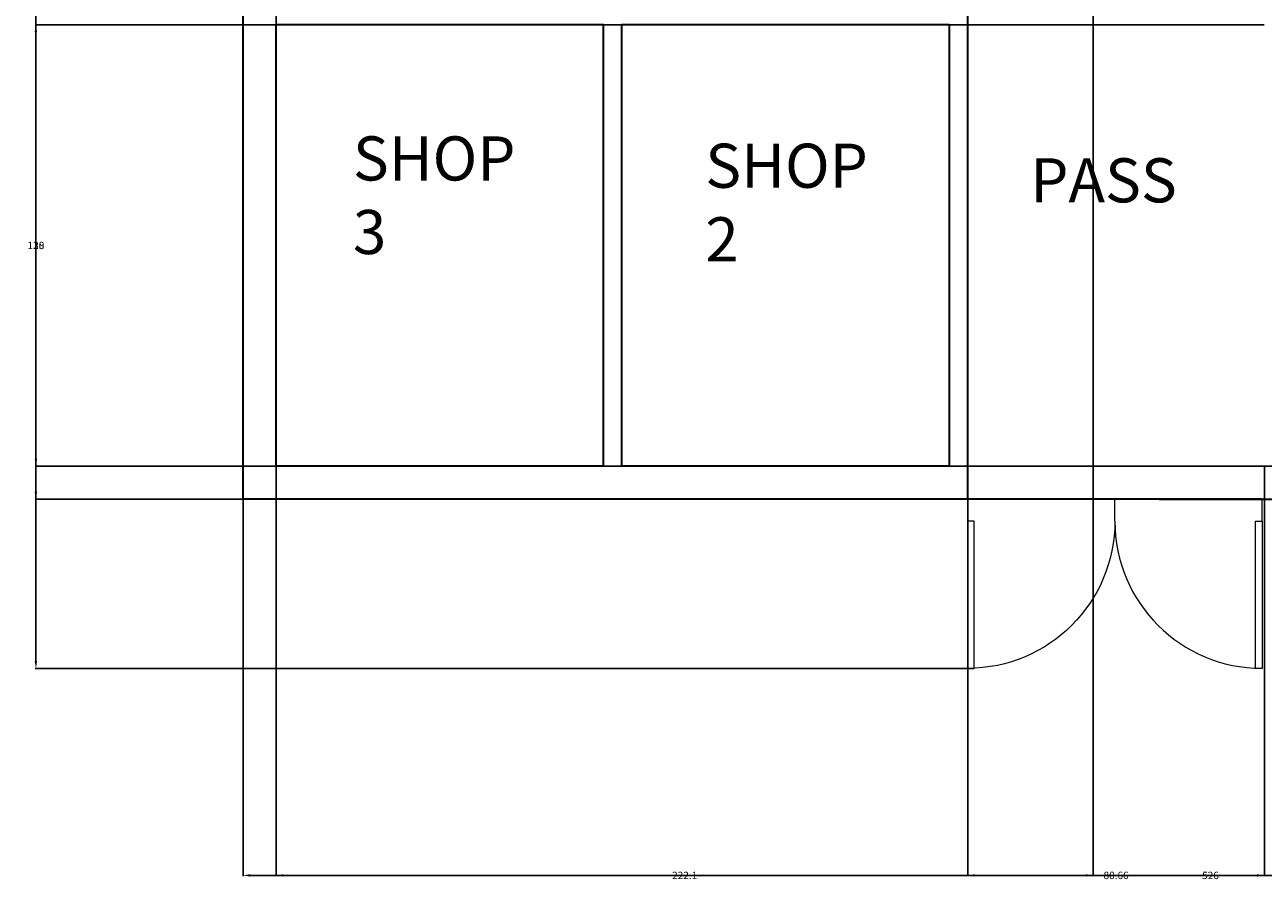
# Model space of a CAD drawing. Units: inches. Extents: x 190 to 836, y -241 to 999.
# Tile 1 of 9: x 191 to 528, y -241 to -8. Entities that reach past the tile are written whole.
import ezdxf

# ---------------------------------------------------------------- set-up
doc = ezdxf.new("R2010")
doc.units = ezdxf.units.IN
doc.header["$MEASUREMENT"] = 0
for name, color, linetype, lineweight in [('A-ANNO-DIMS', 2, 'Continuous', 18), ('A-AREA-IDEN', 7, 'Continuous', 18), ('A-DOOR', 3, 'Continuous', 18), ('A-WALL', 7, 'Continuous', 35)]:
    doc.layers.add(name, color=color, linetype=linetype, lineweight=lineweight)
doc.styles.get("Standard").update_dxf_attribs({"font": 'arial.ttf'})
doc.dimstyles.get("Standard").update_dxf_attribs({"dimtxt": 2, "dimasz": 2, "dimexe": 0.18, "dimexo": 0.0625, "dimgap": 0.09, "dimtad": 0, "dimtih": 1, "dimtoh": 1, "dimdec": 0, "dimzin": 0, "dimdsep": 46, "dimlunit": 3, "dimtxsty": 'Standard', "dimcen": 0.09, "dimadec": 0, "dimazin": 0, "dimtfac": 1, "dimtdec": 0, "dimtofl": 0, "dimtmove": 0, "dimatfit": 3, "dimfxl": 1, "dimtolj": 1, "dimtzin": 0, "dimarcsym": 0})

# ---------------------------------------------------------------- blocks, each defined once
blk = doc.blocks.new('*U6')
for p, q in [((-40, 0), (-40, 6)), ((0, 0), (0, 6))]:
    blk.add_line(p, q)
blk.add_lwpolyline([(0, 0), (0, -40), (-1.75, -40), (-1.75, 0)], close=True)
blk.add_arc((0, 0), 40, 180, 270)
blk = doc.blocks.new('*D16')
at = {"layer": 'A-ANNO-DIMS', "color": 0, "lineweight": -2, "transparency": 16777216}
for p, q in [((250.44, -137.53), (250.44, -239.95)), ((776.44, -137.53), (776.44, -239.95)), ((252.44, -239.77), (511.14, -239.77)), ((774.44, -239.77), (515.74, -239.77))]:
    blk.add_line(p, q, dxfattribs=at)
at = {"layer": 'A-ANNO-DIMS', "color": 0, "transparency": 16777216}
for points in [[(252.44, -239.44), (252.44, -240.11), (250.44, -239.77)], [(774.44, -239.44), (774.44, -240.11), (776.44, -239.77)]]:
    blk.add_solid(points, dxfattribs=at)
at = {"layer": 'Defpoints', "color": 0, "transparency": 16777216}
for p in [(250.44, -137.47), (776.44, -137.47), (776.44, -239.77)]:
    blk.add_point(p, dxfattribs=at)
at = {"layer": 'A-ANNO-DIMS', "color": 0, "transparency": 16777216, "insert": (513.44, -239.77), "char_height": 2, "attachment_point": 5}
blk.add_mtext('\\A1;526', dxfattribs=at)
blk = doc.blocks.new('*D17')
at = {"layer": 'A-ANNO-DIMS', "color": 0, "lineweight": -2, "transparency": 16777216}
for p, q in [((250.38, 941.53), (193.96, 941.53)), ((194.14, 939.53), (194.14, 380.14)), ((194.14, -181.47), (194.14, 377.92)), ((447.38, -183.47), (193.96, -183.47))]:
    blk.add_line(p, q, dxfattribs=at)
at = {"layer": 'A-ANNO-DIMS', "color": 0, "transparency": 16777216}
for points in [[(193.8, 939.53), (194.47, 939.53), (194.14, 941.53)], [(193.8, -181.47), (194.47, -181.47), (194.14, -183.47)]]:
    blk.add_solid(points, dxfattribs=at)
at = {"layer": 'Defpoints', "color": 0, "transparency": 16777216}
for p in [(194.14, 941.53), (250.44, 941.53), (447.44, -183.47)]:
    blk.add_point(p, dxfattribs=at)
at = {"layer": 'A-ANNO-DIMS', "color": 0, "transparency": 16777216, "insert": (194.14, 379.03), "char_height": 2, "attachment_point": 5}
blk.add_mtext('\\A1;1125', dxfattribs=at)
blk = doc.blocks.new('*D29')
at = {"layer": 'A-ANNO-DIMS', "color": 0, "lineweight": -2, "transparency": 16777216}
for p, q in [((259.44, 565.47), (259.44, -239.95)), ((481.55, 565.47), (481.55, -239.95)), ((261.44, -239.77), (367.21, -239.77)), ((479.55, -239.77), (373.79, -239.77))]:
    blk.add_line(p, q, dxfattribs=at)
at = {"layer": 'A-ANNO-DIMS', "color": 0, "transparency": 16777216}
for points in [[(261.44, -239.44), (261.44, -240.11), (259.44, -239.77)], [(479.55, -239.44), (479.55, -240.11), (481.55, -239.77)]]:
    blk.add_solid(points, dxfattribs=at)
at = {"layer": 'Defpoints', "color": 0, "transparency": 16777216}
for p in [(259.44, 565.53), (481.55, 565.53), (481.55, -239.77)]:
    blk.add_point(p, dxfattribs=at)
at = {"layer": 'A-ANNO-DIMS', "color": 0, "transparency": 16777216, "insert": (370.5, -239.77), "char_height": 2, "attachment_point": 5}
blk.add_mtext('\\A1;222.1', dxfattribs=at)
blk = doc.blocks.new('*D34')
at = {"layer": 'A-ANNO-DIMS', "color": 0, "lineweight": -2, "transparency": 16777216}
for p, q in [((447.38, 0.53), (193.96, 0.53)), ((194.14, -1.47), (194.14, -67.36)), ((194.14, -135.47), (194.14, -69.58)), ((447.38, -137.47), (193.96, -137.47))]:
    blk.add_line(p, q, dxfattribs=at)
at = {"layer": 'A-ANNO-DIMS', "color": 0, "transparency": 16777216}
for points in [[(193.8, -1.47), (194.47, -1.47), (194.14, 0.53)], [(193.8, -135.47), (194.47, -135.47), (194.14, -137.47)]]:
    blk.add_solid(points, dxfattribs=at)
at = {"layer": 'Defpoints', "color": 0, "transparency": 16777216}
for p in [(194.14, 0.53), (447.44, 0.53), (447.44, -137.47)]:
    blk.add_point(p, dxfattribs=at)
at = {"layer": 'A-ANNO-DIMS', "color": 0, "transparency": 16777216, "insert": (194.14, -68.47), "char_height": 2, "attachment_point": 5}
blk.add_mtext('\\A1;138', dxfattribs=at)
blk = doc.blocks.new('*D37')
at = {"layer": 'A-ANNO-DIMS', "color": 0, "lineweight": -2, "transparency": 16777216}
for p, q in [((528.1, -128.53), (528.1, -239.95)), ((447.44, -137.53), (447.44, -239.95)), ((449.44, -239.77), (484.31, -239.77)), ((526.1, -239.77), (491.24, -239.77))]:
    blk.add_line(p, q, dxfattribs=at)
at = {"layer": 'A-ANNO-DIMS', "color": 0, "transparency": 16777216}
for points in [[(449.44, -239.44), (449.44, -240.11), (447.44, -239.77)], [(526.1, -239.44), (526.1, -240.11), (528.1, -239.77)]]:
    blk.add_solid(points, dxfattribs=at)
at = {"layer": 'Defpoints', "color": 0, "transparency": 16777216}
for p in [(528.1, -128.47), (447.44, -137.47), (528.1, -239.77)]:
    blk.add_point(p, dxfattribs=at)
at = {"layer": 'A-ANNO-DIMS', "color": 0, "transparency": 16777216, "insert": (487.77, -239.77), "char_height": 2, "attachment_point": 5}
blk.add_mtext('\\A1;80.66', dxfattribs=at)
blk = doc.blocks.new('*D40')
at = {"layer": 'A-ANNO-DIMS', "color": 0, "lineweight": -2, "transparency": 16777216}
for p, q in [((528.04, -8.47), (193.96, -8.47)), ((194.14, -10.47), (194.14, -67.36)), ((194.14, -126.47), (194.14, -69.58)), ((533.04, -128.47), (193.96, -128.47))]:
    blk.add_line(p, q, dxfattribs=at)
at = {"layer": 'A-ANNO-DIMS', "color": 0, "transparency": 16777216}
for points in [[(193.8, -10.47), (194.47, -10.47), (194.14, -8.47)], [(193.8, -126.47), (194.47, -126.47), (194.14, -128.47)]]:
    blk.add_solid(points, dxfattribs=at)
at = {"layer": 'Defpoints', "color": 0, "transparency": 16777216}
for p in [(194.14, -8.47), (528.1, -8.47), (533.1, -128.47)]:
    blk.add_point(p, dxfattribs=at)
at = {"layer": 'A-ANNO-DIMS', "color": 0, "transparency": 16777216, "insert": (194.14, -68.47), "char_height": 2, "attachment_point": 5}
blk.add_mtext('\\A1;120', dxfattribs=at)

msp = doc.modelspace()

# ---------------------------------------------------------------- linework, layer by layer
at = {"layer": 'A-WALL'}
for p, q in [((250.4421, -137.4687), (250.4421, 565.5313)), ((447.4421, -137.4687), (447.4421, 0.5313)), ((259.4421, -128.4687), (259.4421, -8.4687)), ((348.4421, -8.4687), (259.4421, -8.4687)), ((348.4421, -128.4687), (348.4421, -8.4687)), ((442.4421, -8.4687), (353.4421, -8.4687)), ((353.4421, -128.4687), (353.4421, -8.4687)), ((442.4421, -128.4687), (442.4421, -8.4687)), ((348.4421, -128.4687), (259.4421, -128.4687)), ((442.4421, -128.4687), (353.4421, -128.4687)), ((527.4421, -137.4687), (250.4421, -137.4687)), ((499.4421, -137.4687), (776.4421, -137.4687))]:
    msp.add_line(p, q, dxfattribs=at)

# ---------------------------------------------------------------- block references
at = {"layer": 'A-DOOR', "xscale": -1}
msp.add_blockref('*U6', (447.4421, -143.4687), dxfattribs=at)
at = {"layer": 'A-DOOR'}
msp.add_blockref('*U6', (527.4421, -143.4687), dxfattribs=at)

# ---------------------------------------------------------------- texts
at = {"layer": 'A-AREA-IDEN', "char_height": 12, "attachment_point": 1}
for s, insert in [('SHOP 3', (280.3017, -38.8184)), ('SHOP 2', (376.1015, -40.8016)), ('PASS', (464.4558, -44.7679))]:
    msp.add_mtext_dynamic_manual_height_columns(s, width=18.36577, gutter_width=1, heights=[0], dxfattribs=dict(at, insert=insert))

# ---------------------------------------------------------------- dimensions: what is measured, and where the dimension line sits
at = {"layer": 'A-ANNO-DIMS'}
for base, p1, p2, picture, middle in [((194.1371, 941.5313), (447.4421, -183.4687), (250.4421, 941.5313), '*D17', (194.1371, 379.0313)), ((194.1371, 0.5313), (447.4421, -137.4687), (447.4421, 0.5313), '*D34', (194.1371, -68.4687)), ((194.1371, -8.4687), (533.0998, -128.4687), (528.0998, -8.4687), '*D40', (194.1371, -68.4687))]:
    dim = msp.add_linear_dim(base=base, p1=p1, p2=p2, angle=90, dimstyle='Standard', override={"dimdec": 0, "dimlfac": 1, "dimrnd": 0, "dimzin": 0, "dimdsep": 46, "dimlunit": 2}, dxfattribs=at)
    dim.commit()
    dim.dimension.update_dxf_attribs({"geometry": picture, "text_midpoint": middle})
for base, p1, p2, override, picture, middle in [((481.5536, -239.7737), (259.4421, 565.5313), (481.5536, 565.5313), {"dimdec": 1, "dimlfac": 1, "dimrnd": 0, "dimzin": 0, "dimdsep": 46, "dimlunit": 2}, '*D29', (370.4979, -239.7737)), ((528.0998, -239.7737), (447.4421, -137.4687), (528.0998, -128.4687), {"dimdec": 2, "dimlfac": 1, "dimrnd": 0, "dimzin": 0, "dimdsep": 46, "dimlunit": 2}, '*D37', (487.771, -239.7737)), ((776.4421, -239.7737), (250.4421, -137.4687), (776.4421, -137.4687), {"dimdec": 0, "dimlfac": 1, "dimrnd": 0, "dimzin": 0, "dimdsep": 46, "dimlunit": 2}, '*D16', (513.4421, -239.7737))]:
    dim = msp.add_linear_dim(base=base, p1=p1, p2=p2, dimstyle='Standard', override=override, dxfattribs=at)
    dim.commit()
    dim.dimension.update_dxf_attribs({"geometry": picture, "text_midpoint": middle})

doc.saveas('drawing.dxf')
